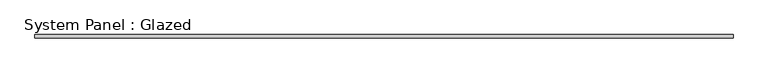
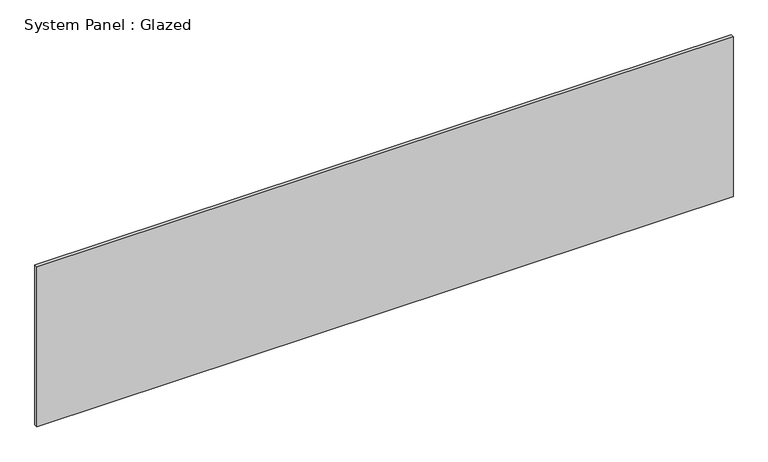
"""IFC4 building model written with IfcOpenShell, lengths in millimetres: plate geometry, System Panel : Glazed."""

from ifc_helpers import new_model, si_unit, origin, origin_with_axes, place, context, project, spatial, polyline, outline, extrude, source, transform, mapped, element, save


def system_panel_glazed_9d7bd240(model_context):
    return source(origin(), model_context, "Body", "SweptSolid", [
        extrude(outline(polyline([(2508.25, 19.05), (-2508.25, 19.05), (-2508.25, 44.45), (2508.25, 44.45), (2508.25, 19.05)])), origin_with_axes(), (0.0, 0.0, 1.0), 1219.2),
    ])


if __name__ == "__main__":
    model = new_model("IFC4")
    model_context = context("Model", 3, world=origin())
    ifc_project = project(units=[si_unit("LENGTHUNIT", "METRE", prefix="MILLI")], contexts=[model_context])
    site = spatial("IfcSite", under=ifc_project)
    building = spatial("IfcBuilding", under=site)
    placement = place(None, origin())
    system_panel_glazed_shape = system_panel_glazed_9d7bd240(model_context)
    element("IfcPlate", 1, ObjectType="System Panel : Glazed", at=placement, inside=building, context=model_context, shape_type="MappedRepresentation", body=[
        mapped(system_panel_glazed_shape, transform((0.0, 0.0, 0.0), x_axis=(1.0, 0.0, 0.0), y_axis=(0.0, 1.0, 0.0), z_axis=(0.0, 0.0, 1.0))),
    ])
    save(model, "model.ifc")

# Revit data of these elements
# Type "System Panel : Glazed"
#   Construction Type Id = "GSP4R"
#   Analytic Construction = "1/8 in Pilkington single glazing"
#   Visual Light Transmittance = 0.9
#   Solar Heat Gain Coefficient = 0.86
#   Heat Transfer Coefficient (U) = 1.18115 BTU/(h·ft²·°F)
# Element 1 (IfcPlate, "System Panel : Glazed")
#   Materials on its faces: "Glass"
# Materials
#   "Glass": class "Glass", colour RGB 0 128 192, transparency 0.75, Description = "Soda Lime Glass", Cost = 0
